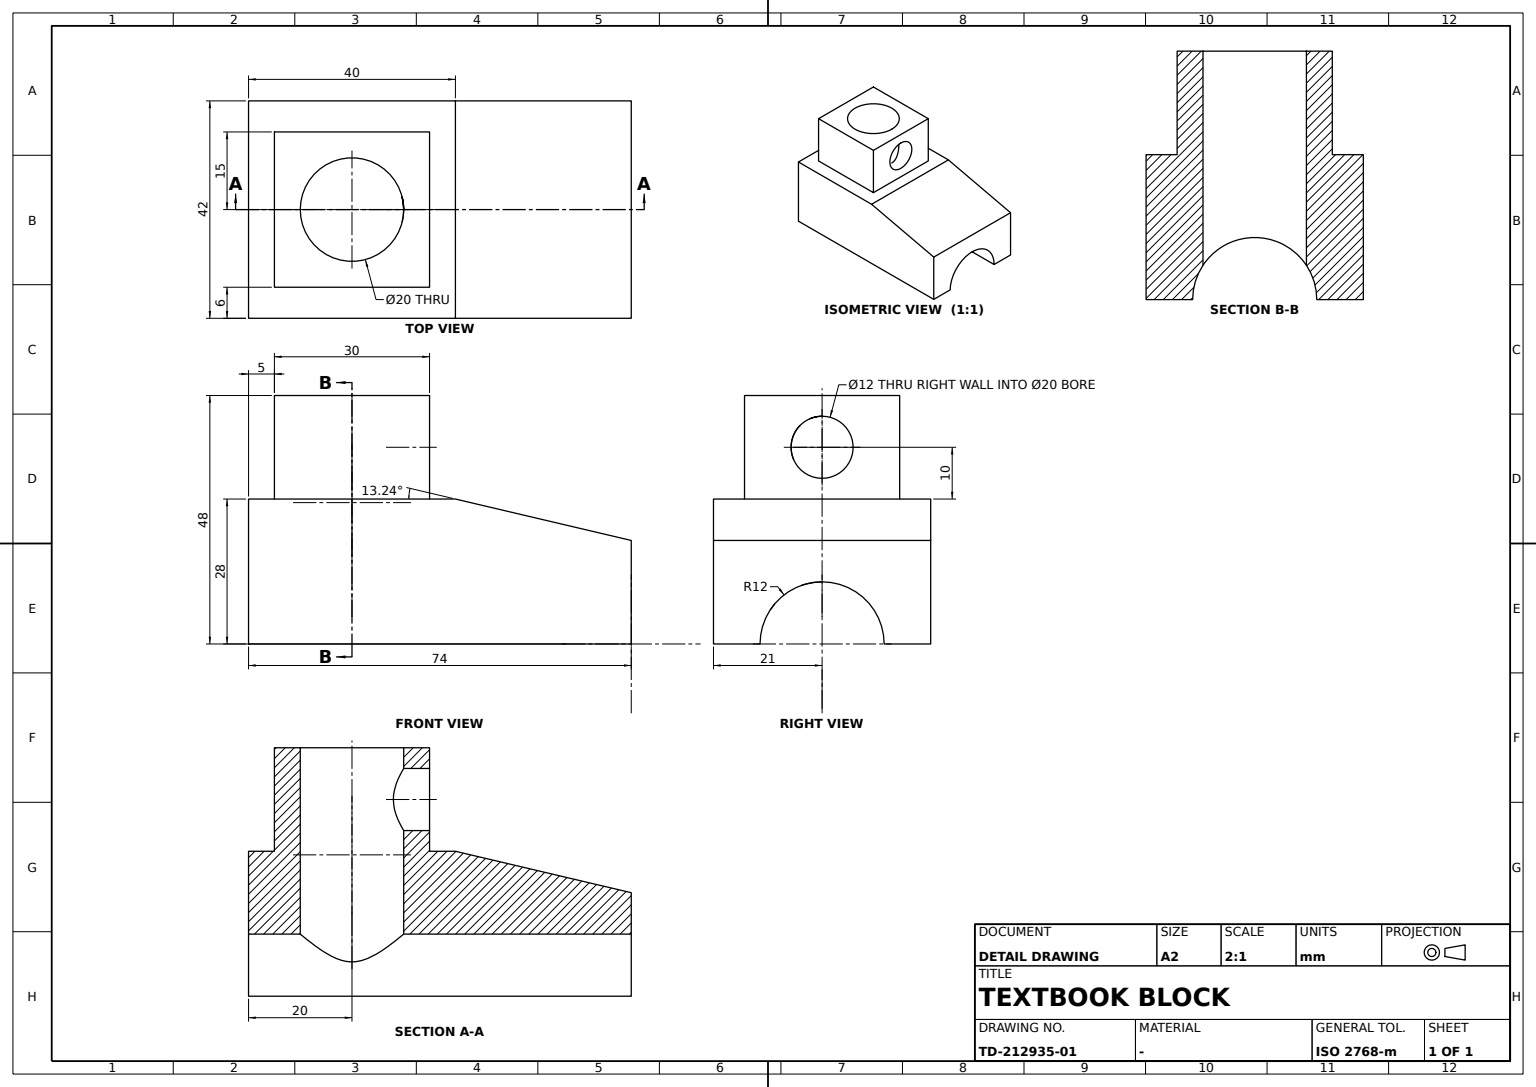
CATIA V5 part; units mm, degrees
sketch "Sketch1" plane through (0, 0, 0) normal (0, 1, 0) x (-1, 0, 0)
  line L0 (0, 0) -> (74, 0)
  line L1 (74, 0) -> (74, 28)
  line L2 (74, 28) -> (34, 28)
  line L3 (34, 28) -> (0, 20)
  point P0 (0, 20)
  line L4 (0, 20) -> (0, 0)
  dimension "length L0" = 74
  dimension "length L2" = 40
  dimension "length L1" = 28
  dimension "length L4" = 20
  constraint horizontal L0 x-axis
  constraint horizontal L2 x-axis
  constraint vertical L1 y-axis
  constraint vertical L4 y-axis
  constraint coincidence P0 y-axis
extrude "Pad1" add sketch "Sketch1" along normal mid plane 42
sketch "Sketch2" plane through (0, 0, 0) normal (1, 0, 0) x (0, 1, 0)
  circle A0 centre (0, 0) radius 12
  dimension "radius A0" = 12
extrude "Pocket1" cut sketch "Sketch2" against normal through all
sketch "Sketch3" plane through (0, 0, 28) normal (0, 0, 1) x (1, 0, 0)
  point P0 (-54, 0)
  line L0 (-39, 15) -> (-39, -15)
  line L1 (-39, -15) -> (-69, -15)
  line L2 (-69, -15) -> (-69, 15)
  line L3 (-69, 15) -> (-39, 15)
  line L4 (-74, -21) -> (-74, 21) construction
  dimension "length L2" = 30
  dimension "length L3" = 30
  dimension "distance L2 L4" = 5
  constraint coincidence P0 x-axis
  constraint vertical L0 y-axis
  constraint vertical L2 y-axis
  constraint horizontal L1 x-axis
  constraint horizontal L3 x-axis
  constraint equidistance L0 L2 P0
  constraint equidistance L1 L3 P0
  constraint symmetry L3 L1 x-axis
extrude "Pad2" add sketch "Sketch3" along normal blind 20
sketch "Sketch4" plane through (0, 0, 48) normal (0, 0, 1) x (1, 0, 0)
  circle A0 centre (-54, 0) radius 10
  point P0 (-54, 0)
  line L0 (-69, 15) -> (-69, -15) construction
  dimension "radius A0" = 10
  dimension "distance L0 P0" = 15
  constraint coincidence P0 x-axis
extrude "Pocket2" cut sketch "Sketch4" against normal through all
sketch "Sketch5" plane through (-39, 0, 0) normal (1, 0, 0) x (0, 1, 0)
  circle A0 centre (0, 38) radius 6
  point P0 (0, 38)
  line L0 (-15, 48) -> (15, 48) construction
  dimension "radius A0" = 6
  dimension "distance P0 L0" = 10
  constraint coincidence P0 y-axis
extrude "Pocket3" cut sketch "Sketch5" against normal up to next
